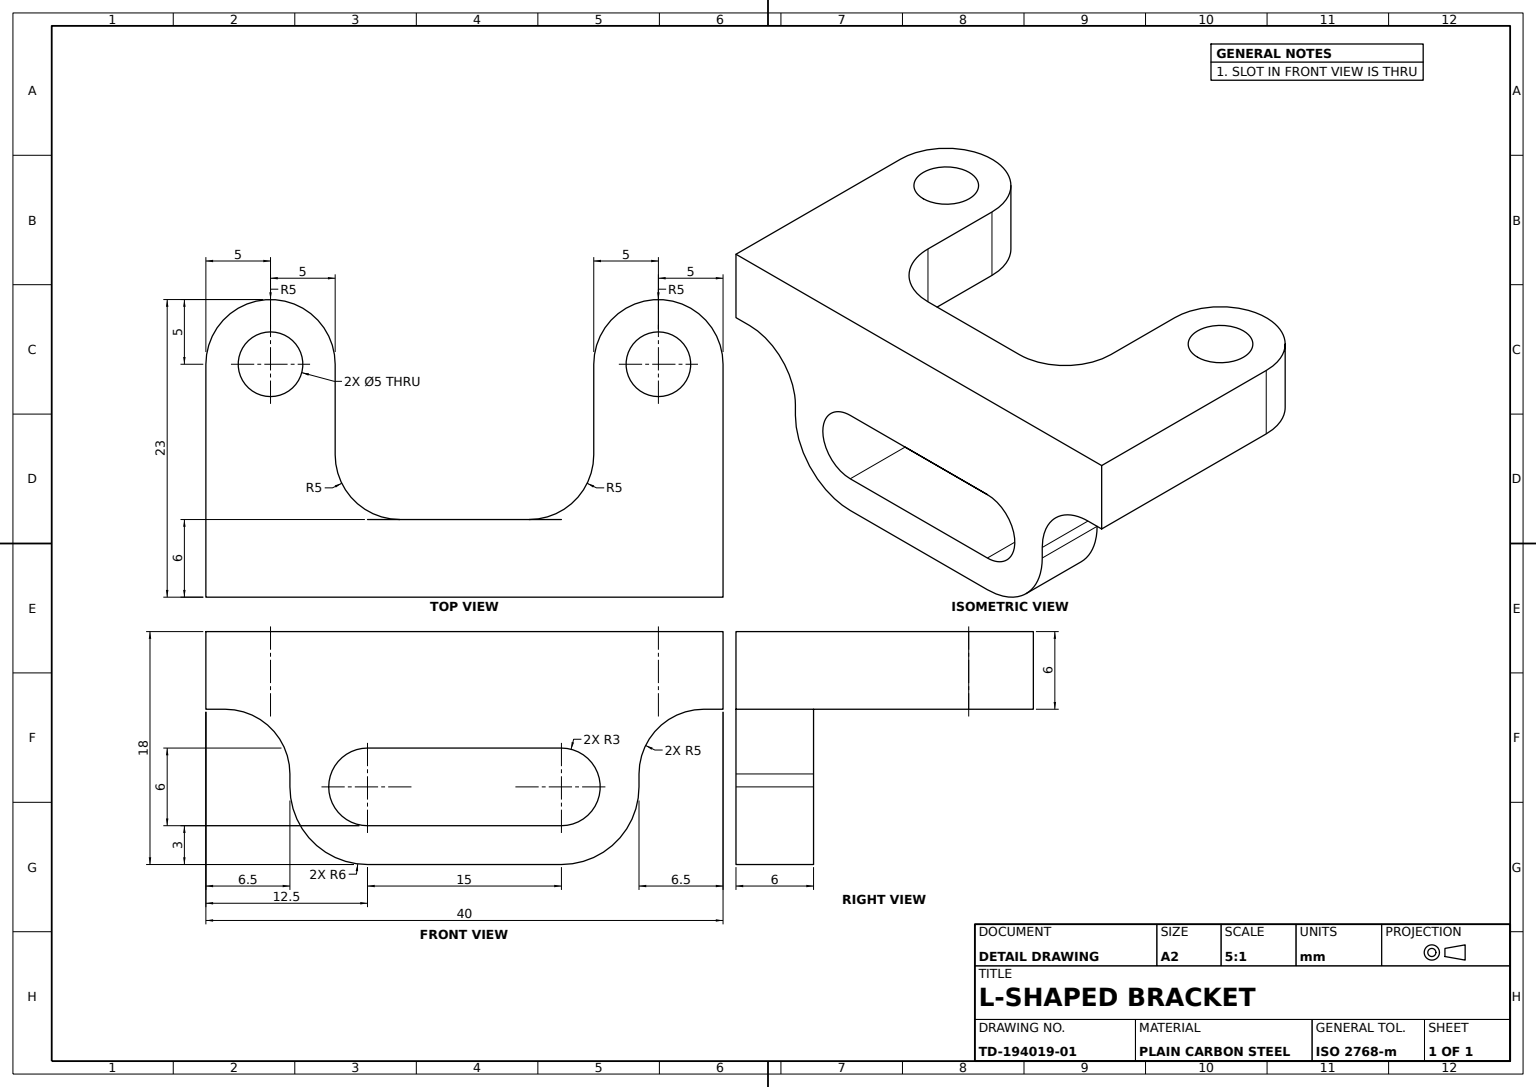
from build123d import *

# Parameters (mm, degrees)
U_BRACKET_BASE_DEPTH    = 6
SLOTTED_TAB_DEPTH       = 6
MOUNTING_HOLES_SKETCH_R = 2.5
MOUNTING_HOLES_2X_DEPTH = 6
TAB_SLOT_DEPTH          = 6


with BuildPart() as part:
    # U Bracket Profile Sketch → U Bracket Base (new body)
    with BuildSketch(Plane.XY):
        with BuildLine():
            Line((0, 0), (40, 0))
            Line((40, 0), (40, -6))
            Line((40, -6), (38.5, -6))
            ThreePointArc((38.5, -6), (34.964466094, -7.464466094), (33.5, -11))
            Line((33.5, -11), (33.5, -12))
            ThreePointArc((33.5, -12), (31.742640687, -16.242640687), (27.5, -18))
            Line((27.5, -18), (12.5, -18))
            ThreePointArc((12.5, -18), (8.257359313, -16.242640687), (6.5, -12))
            Line((6.5, -12), (6.5, -11))
            ThreePointArc((6.5, -11), (5.035533906, -7.464466094), (1.5, -6))
            Line((1.5, -6), (0, -6))
            Line((0, -6), (0, 0))
        make_face()
    extrude(amount=U_BRACKET_BASE_DEPTH)

    # Slotted Tab Sketch → Slotted Tab (add)
    with BuildSketch(Plane(origin=(0, 0, 0), x_dir=(1, 0, 0), z_dir=(0, 1, 0))):
        with BuildLine():
            Line((0, 12), (0, 0))
            Line((0, 0), (15, 0))
            ThreePointArc((15, 0), (11.464466094, 1.464466094), (10, 5))
            Line((10, 5), (10, 12))
            ThreePointArc((10, 12), (5, 17), (0, 12))
        make_face()
        with BuildLine():
            Line((40, 12), (40, 0))
            Line((40, 0), (25, 0))
            ThreePointArc((25, 0), (28.535533906, 1.464466094), (30, 5))
            Line((30, 5), (30, 12))
            ThreePointArc((30, 12), (35, 17), (40, 12))
        make_face()
    extrude(amount=-SLOTTED_TAB_DEPTH)

    # Mounting Holes Sketch → Mounting Holes 2x (cut)
    with BuildSketch(Plane.XZ.offset(6)):
        with Locations(Location((5, -12, 0), (0, 0, 270))):
            Circle(MOUNTING_HOLES_SKETCH_R)
        with Locations(Location((35, -12, 0), (0, 0, 270))):
            Circle(MOUNTING_HOLES_SKETCH_R)
    extrude(amount=-MOUNTING_HOLES_2X_DEPTH, mode=Mode.SUBTRACT)

    # Tab Slot Sketch → Tab Slot (cut)
    with BuildSketch(Plane(origin=(0, 0, 0), x_dir=(-1, 0, 0), z_dir=(0, 0, -1))):
        with BuildLine():
            Line((-27.5, -9), (-12.5, -9))
            ThreePointArc((-12.5, -9), (-9.5, -12), (-12.5, -15))
            Line((-12.5, -15), (-27.5, -15))
            ThreePointArc((-27.5, -15), (-30.5, -12), (-27.5, -9))
        make_face()
    extrude(amount=-TAB_SLOT_DEPTH, mode=Mode.SUBTRACT)


solid = part.part
